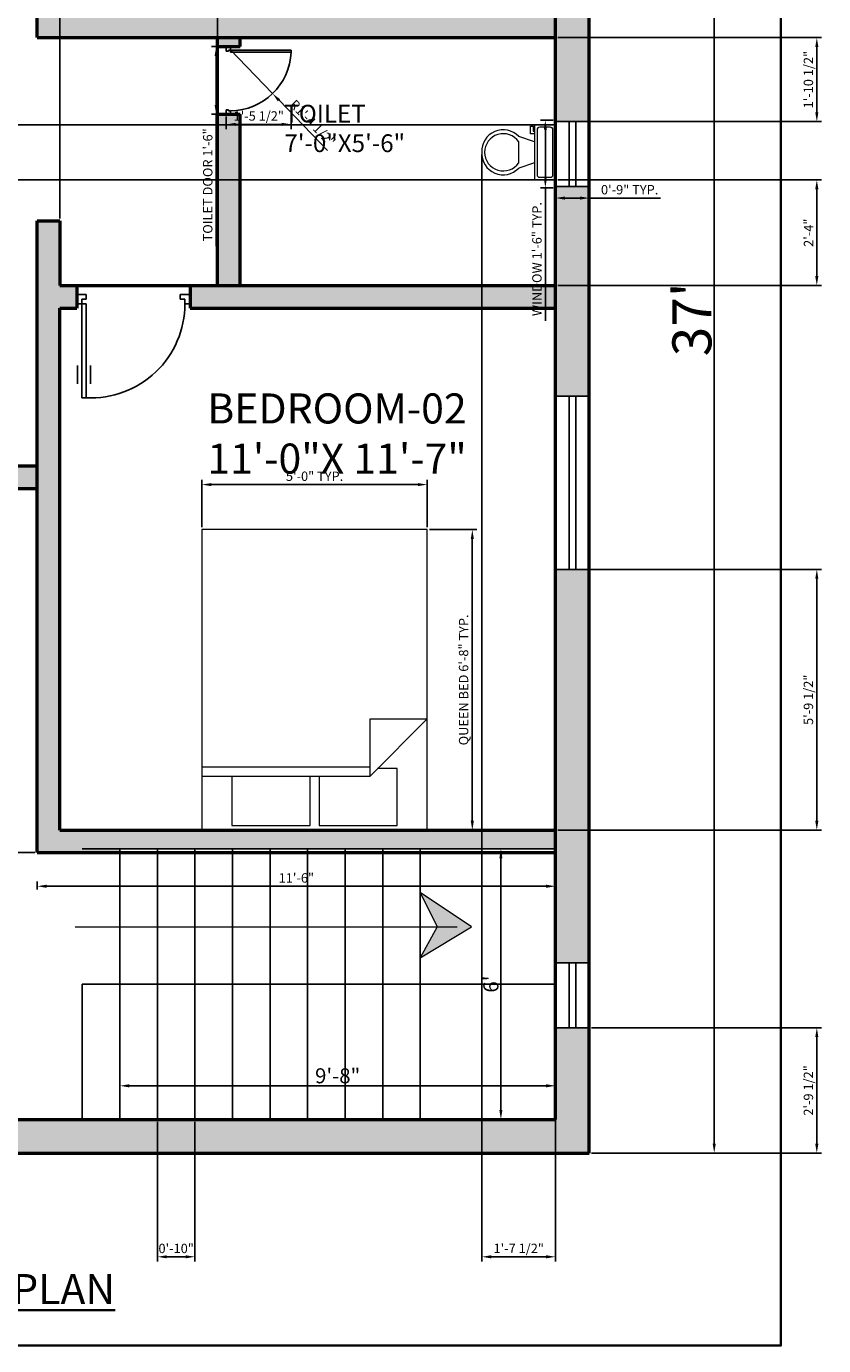
# Model space of a CAD drawing. Units: inches. Extents: x -36 to 398, y -51 to 516.
# Tile 2 of 3: x 186 to 398, y -51 to 300. Entities that reach past the tile are written whole.
import ezdxf

# ---------------------------------------------------------------- set-up
doc = ezdxf.new("R2010")
doc.units = ezdxf.units.IN
doc.header["$PDMODE"] = 34
for name, color, linetype, lineweight in [('A-ANNO-DIMS', 2, 'Continuous', 18), ('A-ANNO-SYMB', 7, 'Continuous', 18), ('A-ANNO-SYMB-PATT', 8, 'Continuous', 13), ('A-ANNO-TTLB', 7, 'Continuous', 35), ('A-AREA-IDEN', 7, 'Continuous', 25), ('A-DOOR', 170, 'Continuous', 25), ('A-FLOR-FIXT', 8, 'Continuous', 18), ('A-FURN', 8, 'Continuous', 18), ('WALL', 7, 'Continuous', 50), ('WINDOW', 5, 'Continuous', 25)]:
    doc.layers.add(name, color=color, linetype=linetype, lineweight=lineweight)
doc.layers.add('A-FLOR-STRS', color=30, linetype='Continuous', lineweight=25, true_color=0xf26722)
doc.layers.add('A-WALL-PATT', color=251, linetype='Continuous', lineweight=13, true_color=0x636466)
doc.styles.get("Standard").update_dxf_attribs({"font": 'arial.ttf'})
doc.dimstyles.new('ISO-25', dxfattribs={"dimtxt": 2.5, "dimasz": 2.5, "dimexe": 1.25, "dimexo": 0.625, "dimtad": 1, "dimdec": 1, "dimlunit": 3, "dimtxsty": 'Standard', "dimcen": 2.5, "dimadec": 0, "dimazin": 0, "dimtfac": 1, "dimtdec": 1, "dimtmove": 0, "dimatfit": 3, "dimfxl": 1, "dimarcsym": 0})

# ---------------------------------------------------------------- blocks, each defined once
blk = doc.blocks.new('WD_00_X1')
for p, q in [((-0.5, 0.5), (0.5, 0.5)), ((-0.48, 0.5), (-0.48, -0.5)), ((0.48, 0.5), (0.48, -0.5)), ((0.48, 0.1), (-0.48, 0.1)), ((0.48, -0.1), (-0.48, -0.1)), ((-0.5, -0.5), (0.5, -0.5))]:
    blk.add_line(p, q)
blk = doc.blocks.new('DR_UKF1')
for p, q in [((-0.458, 0.042), (-0.458, 0.875)), ((-0.458, 0.875), (-0.417, 0.875)), ((-0.417, 0.875), (-0.417, 0.042)), ((-0.494, 0.751), (-0.494, 0.59)), ((-0.381, 0.751), (-0.381, 0.59)), ((-0.5, -0.042), (-0.5, 0.042)), ((-0.5, 0.042), (-0.458, 0.042)), ((-0.417, 0.042), (-0.458, 0.042)), ((-0.458, 0.042), (-0.458, 0)), ((-0.458, 0), (-0.417, 0)), ((-0.417, 0), (-0.417, -0.042)), ((0.417, 0), (0.417, -0.042)), ((0.458, 0), (0.417, 0)), ((0.458, 0.042), (0.458, 0)), ((0.5, 0.042), (0.458, 0.042)), ((0.5, -0.042), (0.5, 0.042)), ((-0.417, -0.042), (-0.5, -0.042)), ((-0.5, -0.042), (-0.5, -0.042)), ((0.417, -0.042), (0.5, -0.042)), ((0.5, -0.042), (0.5, -0.042))]:
    blk.add_line(p, q)
blk.add_arc((-0.375, 0.043), 0.833, 359.9283, 92.866)
blk = doc.blocks.new('DR_D01')
for p, q in [((-0.45, 0.93), (-0.42, 0.93)), ((-0.45, 0.03), (-0.45, 0.93)), ((-0.42, 0.03), (-0.42, 0.93)), ((-0.5, 0.03), (-0.42, 0.03)), ((-0.5, 0.03), (-0.5, -0.03)), ((-0.45, 0.03), (-0.45, 0)), ((-0.45, 0), (-0.435, 0)), ((-0.435, 0), (-0.435, -0.03)), ((0.435, 0), (0.435, -0.03)), ((0.45, 0), (0.435, 0)), ((0.45, 0.03), (0.45, 0)), ((0.5, 0.03), (0.45, 0.03)), ((0.5, -0.03), (0.5, 0.03)), ((-0.435, -0.03), (-0.5, -0.03)), ((0.435, -0.03), (0.5, -0.03))]:
    blk.add_line(p, q)
blk.add_arc((-0.46, 0.021), 0.91, 0.5915, 87.4664)
blk = doc.blocks.new('*U8')
for p, q in [((9.5, -6), (9.5, -2)), ((-10, -8.5), (-8, -8.5)), ((-10, -9.5), (-10, -8.5)), ((-7, -9.5), (-10, -9.5)), ((-8, -8.5), (-8, -8)), ((-7, -8), (-7, -9.5)), ((-4, -8), (-6, -14)), ((4, -8), (6, -14)), ((4, -14), (-4, -14))]:
    blk.add_line(p, q)
blk.add_lwpolyline([(10.5, -8), (10.5, 0), (-10.5, 0), (-10.5, -8)], close=True)
for points in [[(-9.5, -2), (-9.5, -6)], [(8.5, -1), (-8.5, -1)], [(-8.5, -7), (8.5, -7)]]:
    blk.add_lwpolyline(points)
for centre, radius, start, end in [((-8.625, -1.875), 0.8839, 81.8699, 188.1301), ((8.625, -1.875), 0.8839, 351.8699, 98.1301), ((-8.625, -6.125), 0.8839, 171.869898, 278.1301), ((8.625, -6.125), 0.8839, 261.8699, 8.1301), ((-0.4772, -19.9188), 8.0953, 133.01722, 273.38), ((0.0374, -19.8731), 7.127, 124.50543, 269.7), ((-0.0373, -19.8731), 7.127, 270.3, 55.4946), ((0.4773, -19.9188), 8.0953, 266.62, 46.9828)]:
    blk.add_arc(centre, radius, start, end)
blk = doc.blocks.new('Bed - Queen')
for p, q in [((0, -80.00003), (0, 0)), ((0, 0), (59.99999, 0)), ((59.99999, 0), (59.99999, -80.00003)), ((7.99999, -1.2), (28.79998, -1.2)), ((7.99999, -14.4), (7.99999, -1.2)), ((28.79998, -1.2), (28.79998, -14.4)), ((31.19999, -1.2), (51.99999, -1.2)), ((31.19999, -14.4), (31.19999, -1.2)), ((51.99999, -1.2), (51.99999, -16.4)), ((0, -14.4), (44.8, -14.4)), ((44.8, -16.8), (0, -16.8)), ((59.99999, -29.6), (44.8, -14.4)), ((44.8, -14.4), (44.8, -29.6)), ((51.99999, -16.4), (46.79936, -16.4)), ((44.8, -29.6), (59.99999, -29.6)), ((59.99999, -80.00003), (0, -80.00003))]:
    blk.add_line(p, q)
blk = doc.blocks.new('*D11')
at = {"layer": 'A-ANNO-DIMS', "color": 0, "lineweight": -2, "transparency": 16777216}
for p, q in [((210.71, 18.53), (210.71, 19.16)), ((213.21, 17.91), (324.21, 17.91)), ((326.71, 18.53), (326.71, 19.16))]:
    blk.add_line(p, q, dxfattribs=at)
at = {"layer": 'A-ANNO-DIMS', "color": 0, "transparency": 16777216}
for points in [[(213.21, 18.32), (213.21, 17.49), (210.71, 17.91)], [(324.21, 18.32), (324.21, 17.49), (326.71, 17.91)]]:
    blk.add_solid(points, dxfattribs=at)
at = {"layer": 'Defpoints', "color": 0, "transparency": 16777216}
for p in [(210.71, 17.91), (326.71, 17.91), (326.71, 17.91)]:
    blk.add_point(p, dxfattribs=at)
at = {"layer": 'A-ANNO-DIMS', "color": 0, "transparency": 16777216, "insert": (268.71, 20.57), "char_height": 2.5, "attachment_point": 5}
blk.add_mtext('{\\H1.6x;9\'-8"}', dxfattribs=at)
blk = doc.blocks.new('*D12')
at = {"layer": 'A-ANNO-DIMS', "color": 0, "lineweight": -2, "transparency": 16777216}
for p, q in [((314.77, 80.98), (310.93, 80.98)), ((312.18, 78.48), (312.18, 11.48)), ((314.77, 8.98), (310.93, 8.98))]:
    blk.add_line(p, q, dxfattribs=at)
at = {"layer": 'A-ANNO-DIMS', "color": 0, "transparency": 16777216}
for points in [[(311.76, 78.48), (312.59, 78.48), (312.18, 80.98)], [(311.76, 11.48), (312.59, 11.48), (312.18, 8.98)]]:
    blk.add_solid(points, dxfattribs=at)
at = {"layer": 'Defpoints', "color": 0, "transparency": 16777216}
for p in [(315.39, 80.98), (312.18, 8.98), (315.39, 8.98)]:
    blk.add_point(p, dxfattribs=at)
at = {"layer": 'A-ANNO-DIMS', "color": 0, "transparency": 16777216, "insert": (309.51, 44.98), "char_height": 2.5, "attachment_point": 5, "rotation": 90}
blk.add_mtext("{\\H1.6x;6'}", dxfattribs=at)
blk = doc.blocks.new('*D13')
at = {"layer": 'A-ANNO-DIMS', "color": 0, "lineweight": -2, "transparency": 16777216}
for p, q in [((188.71, 70.17), (188.71, 72.28)), ((324.21, 71.03), (191.21, 71.03)), ((326.71, 70.17), (326.71, 72.28))]:
    blk.add_line(p, q, dxfattribs=at)
at = {"layer": 'A-ANNO-DIMS', "color": 0, "transparency": 16777216}
for points in [[(191.21, 71.45), (191.21, 70.62), (188.71, 71.03)], [(324.21, 71.45), (324.21, 70.62), (326.71, 71.03)]]:
    blk.add_solid(points, dxfattribs=at)
at = {"layer": 'Defpoints', "color": 0, "transparency": 16777216}
for p in [(188.71, 71.03), (188.71, 69.55), (326.71, 69.55)]:
    blk.add_point(p, dxfattribs=at)
at = {"layer": 'A-ANNO-DIMS', "color": 0, "transparency": 16777216, "insert": (257.71, 72.93), "char_height": 2.5, "attachment_point": 5}
blk.add_mtext('11\'-6"', dxfattribs=at)
blk = doc.blocks.new('*D14')
at = {"layer": 'A-ANNO-DIMS', "color": 0, "lineweight": -2, "transparency": 16777216}
for p, q in [((188.09, 176.98), (180.39, 176.98)), ((181.64, 174.48), (181.64, 82.48)), ((188.09, 79.98), (180.39, 79.98))]:
    blk.add_line(p, q, dxfattribs=at)
at = {"layer": 'A-ANNO-DIMS', "color": 0, "transparency": 16777216}
for points in [[(181.23, 174.48), (182.06, 174.48), (181.64, 176.98)], [(181.23, 82.48), (182.06, 82.48), (181.64, 79.98)]]:
    blk.add_solid(points, dxfattribs=at)
at = {"layer": 'Defpoints', "color": 0, "transparency": 16777216}
for p in [(188.71, 176.98), (181.64, 79.98), (188.71, 79.98)]:
    blk.add_point(p, dxfattribs=at)
at = {"layer": 'A-ANNO-DIMS', "color": 0, "transparency": 16777216, "insert": (179.74, 128.48), "char_height": 2.5, "attachment_point": 5, "rotation": 90}
blk.add_mtext('8\'-1"', dxfattribs=at)
blk = doc.blocks.new('*D16')
at = {"layer": 'A-ANNO-DIMS', "color": 0, "lineweight": -2, "transparency": 16777216}
for p, q in [((336.34, 443.98), (370.23, 443.98)), ((368.98, 441.48), (368.98, 2.48)), ((336.34, -0.02), (370.23, -0.02))]:
    blk.add_line(p, q, dxfattribs=at)
at = {"layer": 'A-ANNO-DIMS', "color": 0, "transparency": 16777216}
for points in [[(368.56, 441.48), (369.39, 441.48), (368.98, 443.98)], [(368.56, 2.48), (369.39, 2.48), (368.98, -0.02)]]:
    blk.add_solid(points, dxfattribs=at)
at = {"layer": 'Defpoints', "color": 0, "transparency": 16777216}
for p in [(335.71, 443.98), (335.71, -0.02), (368.98, -0.02)]:
    blk.add_point(p, dxfattribs=at)
at = {"layer": 'A-ANNO-DIMS', "color": 0, "transparency": 16777216, "insert": (363.04, 221.98), "char_height": 2.5, "attachment_point": 5, "rotation": 90}
blk.add_mtext("{\\H4.16x;37'}", dxfattribs=at)
blk = doc.blocks.new('STAIR-RISER-PAIR')
for q in [(0, 72), (0, 0)]:
    blk.add_line((0, 36), q)
blk = doc.blocks.new('*D20')
at = {"layer": 'A-ANNO-DIMS', "color": 0, "lineweight": -2, "transparency": 16777216}
for p, q in [((326.09, 274.97), (322.76, 274.97)), ((324.01, 272.47), (324.01, 259.47)), ((326.09, 256.97), (322.76, 256.97)), ((324.01, 256.97), (324.01, 221.58))]:
    blk.add_line(p, q, dxfattribs=at)
at = {"layer": 'A-ANNO-DIMS', "color": 0, "transparency": 16777216}
for points in [[(323.6, 272.47), (324.43, 272.47), (324.01, 274.97)], [(323.6, 259.47), (324.43, 259.47), (324.01, 256.97)]]:
    blk.add_solid(points, dxfattribs=at)
at = {"layer": 'Defpoints', "color": 0, "transparency": 16777216}
for p in [(326.71, 274.97), (324.01, 256.97), (326.71, 256.97)]:
    blk.add_point(p, dxfattribs=at)
at = {"layer": 'A-ANNO-DIMS', "color": 0, "transparency": 16777216, "insert": (322.09, 238.02), "char_height": 2.5, "attachment_point": 5, "rotation": 90}
blk.add_mtext('WINDOW 1\'-6" TYP.', dxfattribs=at)
blk = doc.blocks.new('*D21')
at = {"layer": 'A-ANNO-DIMS', "color": 0, "lineweight": -2, "transparency": 16777216}
for p, q in [((326.71, 256.34), (326.71, 253.02)), ((329.21, 254.27), (333.21, 254.27)), ((335.71, 256.34), (335.71, 253.02)), ((335.71, 254.27), (354.7, 254.27))]:
    blk.add_line(p, q, dxfattribs=at)
at = {"layer": 'A-ANNO-DIMS', "color": 0, "transparency": 16777216}
for points in [[(329.21, 254.68), (329.21, 253.85), (326.71, 254.27)], [(333.21, 254.68), (333.21, 253.85), (335.71, 254.27)]]:
    blk.add_solid(points, dxfattribs=at)
at = {"layer": 'Defpoints', "color": 0, "transparency": 16777216}
for p in [(326.71, 256.97), (335.71, 256.97), (335.71, 254.27)]:
    blk.add_point(p, dxfattribs=at)
at = {"layer": 'A-ANNO-DIMS', "color": 0, "transparency": 16777216, "insert": (346.46, 256.17), "char_height": 2.5, "attachment_point": 5}
blk.add_mtext('0\'-9" TYP.', dxfattribs=at)
blk = doc.blocks.new('*D24')
at = {"layer": 'A-ANNO-DIMS', "color": 0, "lineweight": -2, "transparency": 16777216}
for p, q in [((293.19, 165.98), (305.81, 165.98)), ((304.56, 163.48), (304.56, 88.48)), ((293.19, 85.98), (305.81, 85.98))]:
    blk.add_line(p, q, dxfattribs=at)
at = {"layer": 'A-ANNO-DIMS', "color": 0, "transparency": 16777216}
for points in [[(304.15, 163.48), (304.98, 163.48), (304.56, 165.98)], [(304.15, 88.48), (304.98, 88.48), (304.56, 85.98)]]:
    blk.add_solid(points, dxfattribs=at)
at = {"layer": 'Defpoints', "color": 0, "transparency": 16777216}
for p in [(292.56, 165.98), (292.56, 85.98), (304.56, 85.98)]:
    blk.add_point(p, dxfattribs=at)
at = {"layer": 'A-ANNO-DIMS', "color": 0, "transparency": 16777216, "insert": (302.57, 125.98), "char_height": 2.5, "attachment_point": 5, "rotation": 90}
blk.add_mtext('QUEEN BED 6\'-8" TYP.', dxfattribs=at)
blk = doc.blocks.new('*D25')
at = {"layer": 'A-ANNO-DIMS', "color": 0, "lineweight": -2, "transparency": 16777216}
for p, q in [((232.56, 166.6), (232.56, 179.23)), ((292.56, 166.6), (292.56, 179.23)), ((235.06, 177.98), (290.06, 177.98))]:
    blk.add_line(p, q, dxfattribs=at)
at = {"layer": 'A-ANNO-DIMS', "color": 0, "transparency": 16777216}
for points in [[(235.06, 178.39), (235.06, 177.56), (232.56, 177.98)], [(290.06, 178.39), (290.06, 177.56), (292.56, 177.98)]]:
    blk.add_solid(points, dxfattribs=at)
at = {"layer": 'Defpoints', "color": 0, "transparency": 16777216}
for p in [(292.56, 177.98), (232.56, 165.98), (292.56, 165.98)]:
    blk.add_point(p, dxfattribs=at)
at = {"layer": 'A-ANNO-DIMS', "color": 0, "transparency": 16777216, "insert": (262.56, 179.88), "char_height": 2.5, "attachment_point": 5}
blk.add_mtext('5\'-0" TYP.', dxfattribs=at)
blk = doc.blocks.new('*D26')
at = {"layer": 'A-ANNO-DIMS', "color": 0, "lineweight": -2, "transparency": 16777216}
for p, q in [((238.43, 294.58), (235.11, 294.58)), ((236.36, 292.08), (236.36, 279.08)), ((238.43, 276.58), (235.11, 276.58)), ((236.36, 276.58), (236.36, 241.48))]:
    blk.add_line(p, q, dxfattribs=at)
at = {"layer": 'A-ANNO-DIMS', "color": 0, "transparency": 16777216}
for points in [[(235.94, 292.08), (236.77, 292.08), (236.36, 294.58)], [(235.94, 279.08), (236.77, 279.08), (236.36, 276.58)]]:
    blk.add_solid(points, dxfattribs=at)
at = {"layer": 'Defpoints', "color": 0, "transparency": 16777216}
for p in [(239.06, 294.58), (236.36, 276.58), (239.06, 276.58)]:
    blk.add_point(p, dxfattribs=at)
at = {"layer": 'A-ANNO-DIMS', "color": 0, "transparency": 16777216, "insert": (234.44, 257.78), "char_height": 2.5, "attachment_point": 5, "rotation": 90}
blk.add_mtext('TOILET DOOR 1\'-6"', dxfattribs=at)
blk = doc.blocks.new('*D27')
at = {"layer": 'A-ANNO-DIMS', "color": 0, "lineweight": -2, "transparency": 16777216}
for p, q in [((239.06, 275.96), (239.06, 272.63)), ((256.34, 275.96), (256.34, 272.63)), ((241.56, 273.88), (253.84, 273.88))]:
    blk.add_line(p, q, dxfattribs=at)
at = {"layer": 'A-ANNO-DIMS', "color": 0, "transparency": 16777216}
for points in [[(241.56, 274.3), (241.56, 273.47), (239.06, 273.88)], [(253.84, 274.3), (253.84, 273.47), (256.34, 273.88)]]:
    blk.add_solid(points, dxfattribs=at)
at = {"layer": 'Defpoints', "color": 0, "transparency": 16777216}
for p in [(239.06, 276.58), (256.34, 276.58), (256.34, 273.88)]:
    blk.add_point(p, dxfattribs=at)
at = {"layer": 'A-ANNO-DIMS', "color": 0, "transparency": 16777216, "insert": (247.7, 275.8), "char_height": 2.5, "attachment_point": 5}
blk.add_mtext('1\'-5 1/2"', dxfattribs=at)
blk = doc.blocks.new('*D34')
at = {"layer": 'A-ANNO-DIMS', "color": 0, "lineweight": -2, "transparency": 16777216}
for p, q in [((220.71, 8.35), (220.71, -28.87)), ((230.71, 8.35), (230.71, -28.87)), ((223.21, -27.62), (228.21, -27.62))]:
    blk.add_line(p, q, dxfattribs=at)
at = {"layer": 'A-ANNO-DIMS', "color": 0, "transparency": 16777216}
for points in [[(223.21, -27.21), (223.21, -28.04), (220.71, -27.62)], [(228.21, -27.21), (228.21, -28.04), (230.71, -27.62)]]:
    blk.add_solid(points, dxfattribs=at)
at = {"layer": 'Defpoints', "color": 0, "transparency": 16777216}
for p in [(220.71, 8.98), (230.71, 8.98), (230.71, -27.62)]:
    blk.add_point(p, dxfattribs=at)
at = {"layer": 'A-ANNO-DIMS', "color": 0, "transparency": 16777216, "insert": (225.71, -25.72), "char_height": 2.5, "attachment_point": 5}
blk.add_mtext('0\'-10"', dxfattribs=at)
blk = doc.blocks.new('*D42')
at = {"layer": 'A-ANNO-DIMS', "color": 0, "lineweight": -2, "transparency": 16777216}
for p, q in [((327.34, 296.98), (397.55, 296.98)), ((396.3, 294.48), (396.3, 277.11)), ((327.34, 274.61), (397.55, 274.61))]:
    blk.add_line(p, q, dxfattribs=at)
at = {"layer": 'A-ANNO-DIMS', "color": 0, "transparency": 16777216}
for points in [[(395.88, 294.48), (396.71, 294.48), (396.3, 296.98)], [(395.88, 277.11), (396.71, 277.11), (396.3, 274.61)]]:
    blk.add_solid(points, dxfattribs=at)
at = {"layer": 'Defpoints', "color": 0, "transparency": 16777216}
for p in [(326.71, 296.98), (326.71, 274.61), (396.3, 274.61)]:
    blk.add_point(p, dxfattribs=at)
at = {"layer": 'A-ANNO-DIMS', "color": 0, "transparency": 16777216, "insert": (394.38, 285.79), "char_height": 2.5, "attachment_point": 5, "rotation": 90}
blk.add_mtext('1\'-10 1/2"', dxfattribs=at)
blk = doc.blocks.new('*D43')
at = {"layer": 'A-ANNO-DIMS', "color": 0, "lineweight": -2, "transparency": 16777216}
for p, q in [((327.34, 155.4), (397.55, 155.4)), ((396.3, 88.48), (396.3, 152.9)), ((327.34, 85.98), (397.55, 85.98))]:
    blk.add_line(p, q, dxfattribs=at)
at = {"layer": 'A-ANNO-DIMS', "color": 0, "transparency": 16777216}
for points in [[(395.88, 152.9), (396.71, 152.9), (396.3, 155.4)], [(395.88, 88.48), (396.71, 88.48), (396.3, 85.98)]]:
    blk.add_solid(points, dxfattribs=at)
at = {"layer": 'Defpoints', "color": 0, "transparency": 16777216}
for p in [(326.71, 155.4), (396.3, 155.4), (326.71, 85.98)]:
    blk.add_point(p, dxfattribs=at)
at = {"layer": 'A-ANNO-DIMS', "color": 0, "transparency": 16777216, "insert": (394.38, 120.69), "char_height": 2.5, "attachment_point": 5, "rotation": 90}
blk.add_mtext('5\'-9 1/2"', dxfattribs=at)
blk = doc.blocks.new('*D44')
at = {"layer": 'A-ANNO-DIMS', "color": 0, "lineweight": -2, "transparency": 16777216}
for p, q in [((336.34, 33.37), (397.55, 33.37)), ((396.3, 2.48), (396.3, 30.87)), ((336.34, -0.02), (397.55, -0.02))]:
    blk.add_line(p, q, dxfattribs=at)
at = {"layer": 'A-ANNO-DIMS', "color": 0, "transparency": 16777216}
for points in [[(395.88, 30.87), (396.71, 30.87), (396.3, 33.37)], [(395.88, 2.48), (396.71, 2.48), (396.3, -0.02)]]:
    blk.add_solid(points, dxfattribs=at)
at = {"layer": 'Defpoints', "color": 0, "transparency": 16777216}
for p in [(335.71, 33.37), (396.3, 33.37), (335.71, -0.02)]:
    blk.add_point(p, dxfattribs=at)
at = {"layer": 'A-ANNO-DIMS', "color": 0, "transparency": 16777216, "insert": (394.38, 16.67), "char_height": 2.5, "attachment_point": 5, "rotation": 90}
blk.add_mtext('2\'-9 1/2"', dxfattribs=at)
blk = doc.blocks.new('*D47')
at = {"layer": 'A-ANNO-DIMS', "color": 0, "lineweight": -2, "transparency": 16777216}
for p, q in [((307.12, 265.83), (307.12, -28.87)), ((326.71, 258.48), (326.71, -28.87)), ((309.62, -27.62), (324.21, -27.62))]:
    blk.add_line(p, q, dxfattribs=at)
at = {"layer": 'A-ANNO-DIMS', "color": 0, "transparency": 16777216}
for points in [[(309.62, -27.21), (309.62, -28.04), (307.12, -27.62)], [(324.21, -27.21), (324.21, -28.04), (326.71, -27.62)]]:
    blk.add_solid(points, dxfattribs=at)
at = {"layer": 'Defpoints', "color": 0, "transparency": 16777216}
for p in [(307.12, 266.45), (326.71, 259.1), (326.71, -27.62)]:
    blk.add_point(p, dxfattribs=at)
at = {"layer": 'A-ANNO-DIMS', "color": 0, "transparency": 16777216, "insert": (316.92, -25.71), "char_height": 2.5, "attachment_point": 5}
blk.add_mtext('1\'-7 1/2"', dxfattribs=at)
blk = doc.blocks.new('*D48')
at = {"layer": 'A-ANNO-DIMS', "color": 0, "lineweight": -2, "transparency": 16777216}
for p, q in [((326.09, 273.8), (-17.14, 273.8)), ((-15.89, 271.3), (-15.89, 261.6)), ((326.09, 259.1), (-17.14, 259.1))]:
    blk.add_line(p, q, dxfattribs=at)
at = {"layer": 'A-ANNO-DIMS', "color": 0, "transparency": 16777216}
for points in [[(-16.3, 271.3), (-15.47, 271.3), (-15.89, 273.8)], [(-16.3, 261.6), (-15.47, 261.6), (-15.89, 259.1)]]:
    blk.add_solid(points, dxfattribs=at)
at = {"layer": 'Defpoints', "color": 0, "transparency": 16777216}
for p in [(326.71, 273.8), (-15.89, 259.1), (326.71, 259.1)]:
    blk.add_point(p, dxfattribs=at)
at = {"layer": 'A-ANNO-DIMS', "color": 0, "transparency": 16777216, "insert": (-17.8, 266.45), "char_height": 2.5, "attachment_point": 5, "rotation": 90}
blk.add_mtext('1\'-2 1/2"', dxfattribs=at)
blk = doc.blocks.new('*D49')
at = {"layer": 'A-ANNO-DIMS', "color": 0, "lineweight": -2, "transparency": 16777216}
for p, q in [((327.34, 259.1), (397.55, 259.1)), ((396.3, 233.48), (396.3, 256.6)), ((327.34, 230.98), (397.55, 230.98))]:
    blk.add_line(p, q, dxfattribs=at)
at = {"layer": 'A-ANNO-DIMS', "color": 0, "transparency": 16777216}
for points in [[(395.88, 256.6), (396.71, 256.6), (396.3, 259.1)], [(395.88, 233.48), (396.71, 233.48), (396.3, 230.98)]]:
    blk.add_solid(points, dxfattribs=at)
at = {"layer": 'Defpoints', "color": 0, "transparency": 16777216}
for p in [(326.71, 259.1), (396.3, 259.1), (326.71, 230.98)]:
    blk.add_point(p, dxfattribs=at)
at = {"layer": 'A-ANNO-DIMS', "color": 0, "transparency": 16777216, "insert": (394.42, 245.04), "char_height": 2.5, "attachment_point": 5, "rotation": 90}
blk.add_mtext('2\'-4"', dxfattribs=at)
blk = doc.blocks.new('*D50')
at = {"layer": 'A-ANNO-DIMS', "color": 0, "lineweight": -2, "transparency": 16777216}
for p, q in [((194.71, 248.83), (194.71, 472.83)), ((197.21, 471.58), (234.21, 471.58)), ((236.71, 277.21), (236.71, 472.83))]:
    blk.add_line(p, q, dxfattribs=at)
at = {"layer": 'A-ANNO-DIMS', "color": 0, "transparency": 16777216}
for points in [[(197.21, 471.99), (197.21, 471.16), (194.71, 471.58)], [(234.21, 471.99), (234.21, 471.16), (236.71, 471.58)]]:
    blk.add_solid(points, dxfattribs=at)
at = {"layer": 'Defpoints', "color": 0, "transparency": 16777216}
for p in [(236.71, 471.58), (236.71, 276.58), (194.71, 248.21)]:
    blk.add_point(p, dxfattribs=at)
at = {"layer": 'A-ANNO-DIMS', "color": 0, "transparency": 16777216, "insert": (215.71, 473.48), "char_height": 2.5, "attachment_point": 5}
blk.add_mtext('3\'-6"', dxfattribs=at)
blk = doc.blocks.new('*D52')
at = {"layer": 'A-ANNO-DIMS', "color": 0, "lineweight": -2, "transparency": 16777216}
for p, q in [((239.97, 293.87), (251.36, 282.09)), ((266.03, 266.91), (253.09, 280.29))]:
    blk.add_line(p, q, dxfattribs=at)
at = {"layer": 'A-ANNO-DIMS', "color": 0, "transparency": 16777216}
blk.add_solid([(253.39, 280.58), (252.79, 280), (251.36, 282.09)], dxfattribs=at)
at = {"layer": 'Defpoints', "color": 0, "transparency": 16777216}
for p in [(239.97, 293.87), (251.36, 282.09)]:
    blk.add_point(p, dxfattribs=at)
at = {"layer": 'A-ANNO-DIMS', "color": 0, "transparency": 16777216, "insert": (261.81, 274.03), "char_height": 2.5, "attachment_point": 5, "rotation": 314.028}
blk.add_mtext('R1\'-4 1/2"', dxfattribs=at)

msp = doc.modelspace()

# ---------------------------------------------------------------- hatches: boundary and pattern name
at = {"layer": 'A-ANNO-SYMB-PATT'}
h = msp.add_hatch(color=256, dxfattribs=at)
h.dxf.hatch_style = 1
h.paths.add_polyline_path([(295.23, 60.27), (290.71, 51.99), (304.38, 60.27), (290.71, 69.36)])
at = {"layer": 'A-WALL-PATT'}
h = msp.add_hatch(color=256, dxfattribs=at)
h.dxf.hatch_style = 1
h.paths.add_polyline_path([(335.71, 155.4), (326.71, 155.4), (326.71, 154.44), (326.71, 50.65), (335.71, 50.65), (335.71, 51.01)])
h.paths.add_polyline_path([(335.71, 257.33), (326.71, 257.33), (326.71, 256.97), (326.71, 201.48), (335.71, 201.48), (335.71, 202.44)])
h.paths.add_polyline_path([(335.71, 33.37), (326.71, 33.37), (326.71, 33.01), (326.71, 8.97), (200.71, 8.97), (148.47, 8.97), (148.47, -0.02), (335.71, -0.02)])
h.paths.add_polyline_path([(118.44, 5.24), (118.46, 8.97), (92.19, 8.97), (92.19, -0.02), (93.15, -0.02), (118.46, -0.02), (118.46, 2.74), (118.44, 2.74)])
h.paths.add_polyline_path([(20.71, 85.44), (11.71, 85.44), (11.71, 84.48), (11.71, -0.02), (46.11, -0.02), (46.11, 8.97), (45.15, 8.97), (20.71, 8.97)])
h.paths.add_polyline_path([(20.71, 246.46), (11.71, 246.46), (11.71, 245.5), (11.71, 131.52), (20.71, 131.52), (20.71, 132.48)])
h.paths.add_polyline_path([(152.93, 182.98), (20.71, 182.98), (20.71, 176.98), (152.93, 176.98)])
h.paths.add_polyline_path([(188.71, 182.98), (182.93, 182.98), (182.93, 176.98), (188.71, 176.98)])
h.paths.add_polyline_path([(194.71, 224.98), (199.29, 224.98), (199.29, 230.98), (188.71, 230.98), (188.71, 79.98), (210.71, 79.98), (210.71, 80.98), (326.71, 80.98), (326.71, 85.98), (194.71, 85.98)])
h.paths.add_polyline_path([(326.71, 230.98), (229.41, 230.98), (229.41, 224.98), (326.71, 224.98)], flags=0)
h.paths.add_polyline_path([(242.71, 276.58), (236.71, 276.58), (236.71, 230.98), (242.71, 230.98)])
h.paths.add_polyline_path([(326.71, 302.98), (194.71, 302.98), (194.71, 310.64), (188.71, 310.64), (188.71, 296.98), (326.71, 296.98)])
h.paths.add_polyline_path([(242.71, 296.98), (236.71, 296.98), (236.71, 294.58), (242.71, 294.58)])
h.paths.add_polyline_path([(194.71, 434.98), (188.71, 434.98), (188.71, 340.61), (191.4, 340.61), (191.4, 340.64), (193.9, 340.64), (194.71, 340.61)])
h.paths.add_polyline_path([(335.71, 443.98), (174.69, 443.98), (174.69, 434.98), (175.05, 434.98), (326.71, 434.98), (326.71, 384.97), (335.71, 384.97), (335.71, 385.93)])
h.paths.add_polyline_path([(335.71, 338.89), (326.71, 338.89), (326.71, 337.93), (326.71, 274.61), (335.71, 274.61), (335.71, 274.97)])
h.paths.add_polyline_path([(157.41, 443.98), (157.05, 443.98), (11.71, 443.98), (11.71, 413.15), (20.71, 413.15), (20.71, 414.11), (20.71, 434.98), (157.41, 434.98)])
h.paths.add_polyline_path([(20.71, 367.07), (11.71, 367.07), (11.71, 366.11), (11.71, 292.54), (20.71, 292.54), (20.71, 293.5)])
h = msp.add_hatch(color=256, dxfattribs=at)
h.dxf.hatch_style = 1
h.paths.add_polyline_path([(194.71, 248.21), (188.71, 248.21), (188.71, 230.98), (194.71, 230.98)])
h = msp.add_hatch(color=256, dxfattribs=at)
h.dxf.hatch_style = 1
h.paths.add_polyline_path([(326.71, 224.98), (326.71, 230.98), (229.41, 230.98), (229.41, 224.98)])

# ---------------------------------------------------------------- linework, layer by layer
at = {"layer": 'A-ANNO-SYMB'}
msp.add_line((198.84, 60.27), (300.56, 60.27), dxfattribs=at)
msp.add_lwpolyline([(290.71, 51.99), (304.38, 60.27), (290.71, 69.36), (295.23, 60.27)], close=True, dxfattribs=at)
at = {"layer": 'A-ANNO-TTLB'}
msp.add_lwpolyline([(-35.73, 515.75), (386.76, 515.75), (386.76, -51.27), (-35.73, -51.27)], close=True, dxfattribs=at)
at = {"layer": 'A-FLOR-STRS'}
for p, q in [((200.71, 80.98), (326.71, 80.98)), ((326.71, 80.98), (326.71, 8.97)), ((200.71, 44.98), (200.71, 8.97)), ((200.71, 44.98), (326.71, 44.98)), ((326.71, 8.97), (200.71, 8.97))]:
    msp.add_line(p, q, dxfattribs=at)
at = {"layer": 'WALL'}
for p, q in [((335.71, -0.02), (335.71, 443.98)), ((188.71, 296.98), (188.71, 434.98)), ((326.71, 8.97), (326.71, 434.98)), ((188.71, 296.98), (326.71, 296.98)), ((236.71, 230.98), (236.71, 296.98)), ((242.71, 294.58), (242.71, 296.98)), ((236.71, 294.58), (242.71, 294.58)), ((236.71, 276.58), (242.71, 276.58)), ((242.71, 230.98), (242.71, 276.58)), ((188.71, 230.98), (188.71, 248.21)), ((188.71, 248.21), (194.71, 248.21)), ((194.71, 248.21), (194.71, 230.98)), ((188.71, 79.98), (188.71, 230.98)), ((194.71, 230.98), (326.71, 230.98)), ((199.29, 230.98), (199.29, 224.98)), ((229.41, 230.98), (229.41, 224.98)), ((194.71, 224.98), (199.29, 224.98)), ((194.71, 85.98), (194.71, 224.98)), ((229.41, 224.98), (326.71, 224.98)), ((182.93, 182.98), (188.71, 182.98)), ((20.71, 176.98), (188.71, 176.98)), ((194.71, 85.98), (326.71, 85.98)), ((188.71, 79.98), (326.71, 79.98)), ((148.47, 8.97), (326.71, 8.97)), ((11.71, -0.02), (335.71, -0.02))]:
    msp.add_line(p, q, dxfattribs=at)

# ---------------------------------------------------------------- block references
at = {"layer": 'A-DOOR'}
for name, p, xscale, yscale, zscale, rotation in [('DR_D01', (239.6, 285.58), 18, 18, 18, 269.9999999999883), ('DR_UKF1', (214.29, 227.35), -30, 30, 30, 180)]:
    msp.add_blockref(name, p, dxfattribs=dict(at, xscale=xscale, yscale=yscale, zscale=zscale, rotation=rotation))
at = {"layer": 'A-FLOR-FIXT', "xscale": 0.6997583397893522, "yscale": 0.6997583397893522, "zscale": 0.6997583397893522, "rotation": 269.9999999999998}
msp.add_blockref('*U8', (326.71, 266.45), dxfattribs=at)
at = {"layer": 'A-FLOR-STRS'}
for p in [(210.71, 8.97), (220.71, 8.97), (230.71, 8.97), (240.71, 8.97), (250.71, 8.97), (260.71, 8.97), (270.71, 8.97), (280.71, 8.97), (290.71, 8.97)]:
    msp.add_blockref('STAIR-RISER-PAIR', p, dxfattribs=at)
at = {"layer": 'A-FURN', "xscale": -1, "rotation": 180}
msp.add_blockref('Bed - Queen', (232.56, 85.98), dxfattribs=at)
at = {"layer": 'WINDOW', "yscale": 9}
for p, xscale, zscale, rotation in [((331.21, 265.97), 18, 18, 270), ((331.21, 178.44), 48, 48, 89.99999999999999), ((331.21, 42.01), 18, 18, 270)]:
    msp.add_blockref('WD_00_X1', p, dxfattribs=dict(at, xscale=xscale, zscale=zscale, rotation=rotation))

# ---------------------------------------------------------------- texts
at = {"layer": 'A-ANNO-TTLB', "insert": (96.2, -32.22), "char_height": 8.0065, "attachment_point": 1}
msp.add_mtext_dynamic_manual_height_columns('{\\fArial|b1|i0|c0|p34;\\LGROUND FLOOR PLAN}', width=139.8375, gutter_width=40.03, heights=[0], dxfattribs=at)
at = {"layer": 'A-AREA-IDEN', "attachment_point": 1}
for s, width, gutter_width, insert, char_height in [('TOILET\\P7\'-0"X5\'-6"', 35.7588, 23.61, (254.51, 279.1), 4.7211), ('BEDROOM-02\\P11\'-0"X 11\'-7"', 96.1834, 40.03, (234, 202.25), 8.0065)]:
    msp.add_mtext_dynamic_manual_height_columns(s, width=width, gutter_width=gutter_width, heights=[0], dxfattribs=dict(at, insert=insert, char_height=char_height))

# ---------------------------------------------------------------- dimensions: what is measured, and where the dimension line sits
at = {"layer": 'A-ANNO-DIMS'}
for base, p1, p2, override, picture, middle in [((236.71, 471.58), (194.71, 248.21), (236.71, 276.58), {"dimdec": 1, "dimlfac": 1, "dimrnd": 0, "dimzin": 1, "dimdsep": 46, "dimlunit": 4, "dimfrac": 2}, '*D50', (215.71, 473.48)), ((256.34, 273.88), (239.06, 276.58), (256.34, 276.58), {"dimdec": 1, "dimlfac": 1, "dimrnd": 0, "dimzin": 1, "dimdsep": 46, "dimlunit": 4, "dimfrac": 2}, '*D27', (247.7, 275.8)), ((326.71, -27.62), (307.12, 266.45), (326.71, 259.1), {"dimdec": 1, "dimlfac": 1, "dimrnd": 0, "dimzin": 1, "dimdsep": 46, "dimlunit": 4, "dimfrac": 2}, '*D47', (316.92, -25.71)), ((188.71, 71.03), (326.71, 69.55), (188.71, 69.55), {"dimclrd": 0, "dimclre": 0, "dimclrt": 0}, '*D13', (257.71, 72.93)), ((230.71, -27.62), (220.71, 8.97), (230.71, 8.97), {"dimdec": 1, "dimlfac": 1, "dimrnd": 0, "dimzin": 1, "dimdsep": 46, "dimlunit": 4, "dimfrac": 2}, '*D34', (225.71, -25.72))]:
    dim = msp.add_linear_dim(base=base, p1=p1, p2=p2, dimstyle='ISO-25', override=override, dxfattribs=at)
    dim.commit()
    dim.dimension.update_dxf_attribs({"geometry": picture, "text_midpoint": middle})
for base, p1, p2, angle, text, override, picture, middle in [((368.98, -0.02), (335.71, 443.98), (335.71, -0.02), 90, '{\\H4.16x;<>}', {"dimclrd": 0, "dimclre": 0, "dimclrt": 0}, '*D16', (363.04, 221.98)), ((236.36, 276.58), (239.06, 294.58), (239.06, 276.58), 270, 'TOILET DOOR <>', {"dimdec": 1, "dimlfac": 1, "dimrnd": 0, "dimzin": 1, "dimdsep": 46, "dimlunit": 4, "dimfrac": 2}, '*D26', (234.44, 257.78)), ((324.01, 256.97), (326.71, 274.97), (326.71, 256.97), 270, 'WINDOW <> TYP.', {"dimdec": 1, "dimlfac": 1, "dimrnd": 0, "dimzin": 1, "dimdsep": 46, "dimlunit": 4, "dimfrac": 2}, '*D20', (322.09, 238.02)), ((304.56, 85.98), (292.56, 165.98), (292.56, 85.98), 270, 'QUEEN BED <> TYP.', {"dimdec": 1, "dimlfac": 1, "dimrnd": 0, "dimzin": 1, "dimdsep": 46, "dimlunit": 4, "dimfrac": 2}, '*D24', (302.57, 125.98)), ((312.18, 8.97), (315.39, 80.98), (315.39, 8.97), 90, '{\\H1.6x;<>}', {"dimclrd": 0, "dimclre": 0, "dimclrt": 0}, '*D12', (309.51, 44.98))]:
    dim = msp.add_linear_dim(base=base, p1=p1, p2=p2, angle=angle, text=text, dimstyle='ISO-25', override=override, dxfattribs=at)
    dim.commit()
    dim.dimension.update_dxf_attribs({"geometry": picture, "text_midpoint": middle})
for base, p1, p2, override, picture, middle in [((396.3, 274.61), (326.71, 296.98), (326.71, 274.61), {"dimdec": 1, "dimlfac": 1, "dimrnd": 0, "dimzin": 1, "dimdsep": 46, "dimlunit": 4, "dimfrac": 2}, '*D42', (394.38, 285.79)), ((-15.89, 259.1), (326.71, 273.8), (326.71, 259.1), {"dimdec": 1, "dimlfac": 1, "dimrnd": 0, "dimzin": 1, "dimdsep": 46, "dimlunit": 4, "dimfrac": 2}, '*D48', (-17.8, 266.45)), ((396.3, 259.1), (326.71, 230.98), (326.71, 259.1), {"dimdec": 1, "dimlfac": 1, "dimrnd": 0, "dimzin": 1, "dimdsep": 46, "dimlunit": 4, "dimfrac": 2}, '*D49', (394.42, 245.04)), ((181.64, 79.98), (188.71, 176.98), (188.71, 79.98), {"dimclrd": 0, "dimclre": 0, "dimclrt": 0}, '*D14', (179.74, 128.48)), ((396.3, 155.4), (326.71, 85.98), (326.71, 155.4), {"dimdec": 1, "dimlfac": 1, "dimrnd": 0, "dimzin": 1, "dimdsep": 46, "dimlunit": 4, "dimfrac": 2}, '*D43', (394.38, 120.69)), ((396.3, 33.37), (335.71, -0.02), (335.71, 33.37), {"dimdec": 1, "dimlfac": 1, "dimrnd": 0, "dimzin": 1, "dimdsep": 46, "dimlunit": 4, "dimfrac": 2}, '*D44', (394.38, 16.67))]:
    dim = msp.add_linear_dim(base=base, p1=p1, p2=p2, angle=90, dimstyle='ISO-25', override=override, dxfattribs=at)
    dim.commit()
    dim.dimension.update_dxf_attribs({"geometry": picture, "text_midpoint": middle})
dim = msp.add_radius_dim(center=(239.97, 293.87), mpoint=(251.36, 282.09), dimstyle='ISO-25', override={"dimdec": 1, "dimlfac": 1, "dimrnd": 0, "dimzin": 1, "dimdsep": 46, "dimlunit": 4, "dimfrac": 2}, dxfattribs=at)
dim.commit()
dim.dimension.update_dxf_attribs({"geometry": '*D52', "text_midpoint": (261.81, 274.03)})
for base, p1, p2, text, override, picture, middle in [((335.71, 254.27), (326.71, 256.97), (335.71, 256.97), '<> TYP.', {"dimdec": 1, "dimlfac": 1, "dimrnd": 0, "dimzin": 1, "dimdsep": 46, "dimlunit": 4, "dimfrac": 2}, '*D21', (346.46, 256.17)), ((292.56, 177.98), (232.56, 165.98), (292.56, 165.98), '<> TYP.', {"dimdec": 1, "dimlfac": 1, "dimrnd": 0, "dimzin": 1, "dimdsep": 46, "dimlunit": 4, "dimfrac": 2}, '*D25', (262.56, 179.88)), ((326.71, 17.91), (210.71, 17.91), (326.71, 17.91), '{\\H1.6x;<>}', {"dimclrd": 0, "dimclre": 0, "dimclrt": 0}, '*D11', (268.71, 20.57))]:
    dim = msp.add_linear_dim(base=base, p1=p1, p2=p2, text=text, dimstyle='ISO-25', override=override, dxfattribs=at)
    dim.commit()
    dim.dimension.update_dxf_attribs({"geometry": picture, "text_midpoint": middle})

doc.saveas('drawing.dxf')
